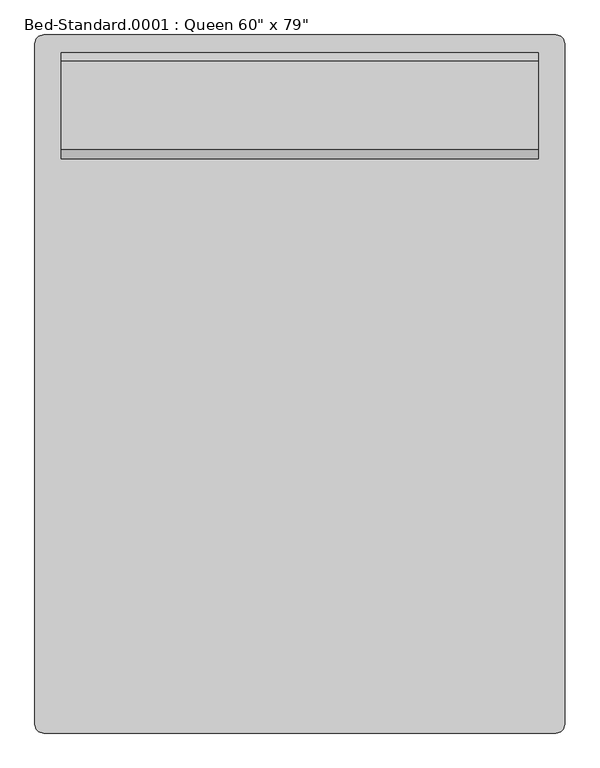
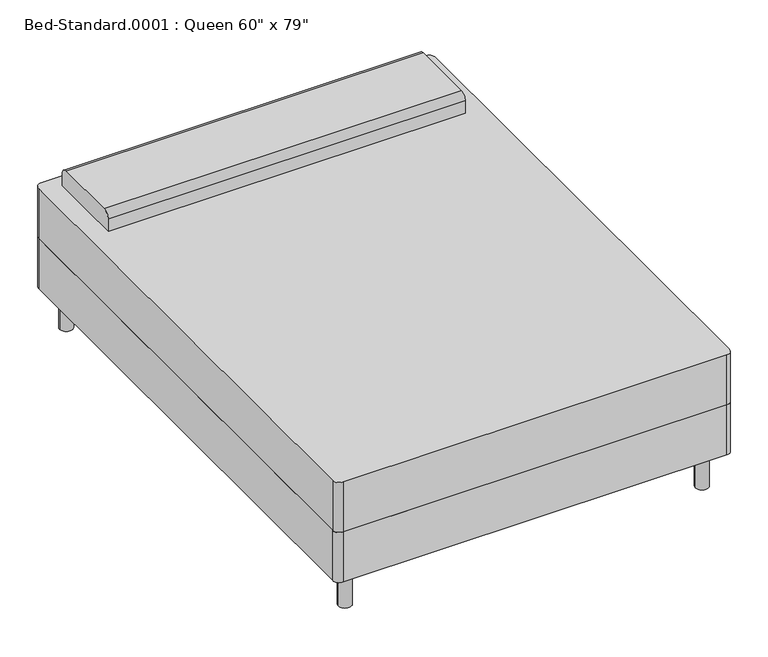
"""IFC4 building model written with IfcOpenShell, lengths in millimetres: furniture geometry."""

from ifc_helpers import new_model, si_unit, point, frame, frame_2d, origin, origin_with_axes, place, context, project, spatial, polyline, circle_curve, trimmed, segment, composite_curve, outline, extrude, source, transform, mapped, element, save


def furniture_e1791683(model_context):
    return source(origin(), model_context, "Body", "SweptSolid", [
        extrude(outline(composite_curve([segment(polyline([(-490.5114754, -1023.495082), (-490.5114754, 932.304918)]), True, "CONTINUOUS"), segment(trimmed(circle_curve(frame_2d((-465.1114754, 932.304918)), 25.4), [point((-490.5114754, 932.304918))], [point((-465.1114754, 957.704918))], False, "CARTESIAN"), True, "CONTINUOUS"), segment(polyline([(-465.1114754, 957.704918), (1008.0885246, 957.704918)]), True, "CONTINUOUS"), segment(trimmed(circle_curve(frame_2d((1008.0885246, 932.304918)), 25.4), [point((1008.0885246, 957.704918))], [point((1033.4885246, 932.304918))], False, "CARTESIAN"), True, "CONTINUOUS"), segment(polyline([(1033.4885246, 932.304918), (1033.4885246, -1023.495082)]), True, "CONTINUOUS"), segment(trimmed(circle_curve(frame_2d((1008.0885246, -1023.495082)), 25.4), [point((1033.4885246, -1023.495082))], [point((1008.0885246, -1048.895082))], False, "CARTESIAN"), True, "CONTINUOUS"), segment(polyline([(1008.0885246, -1048.895082), (-465.1114754, -1048.895082)]), True, "CONTINUOUS"), segment(trimmed(circle_curve(frame_2d((-465.1114754, -1023.495082)), 25.4), [point((-465.1114754, -1048.895082))], [point((-490.5114754, -1023.495082))], False, "CARTESIAN"), True, "CONTINUOUS")], self_intersect=False)), frame((0.0, 0.0, 152.4), z_axis=(0.0, 0.0, 1.0), x_axis=(1.0, 0.0, 0.0)), (0.0, 0.0, 1.0), 203.2),
        extrude(outline(composite_curve([segment(polyline([(602.104918, 558.8), (602.104918, 609.6)]), True, "CONTINUOUS"), segment(trimmed(circle_curve(frame_2d((627.504918, 609.6)), 25.4), [point((602.104918, 609.6))], [point((627.504918, 635.0))], False, "CARTESIAN"), True, "CONTINUOUS"), segment(polyline([(627.504918, 635.0), (881.504918, 635.0)]), True, "CONTINUOUS"), segment(trimmed(circle_curve(frame_2d((881.504918, 609.6)), 25.4), [point((881.504918, 635.0))], [point((906.904918, 609.6))], False, "CARTESIAN"), True, "CONTINUOUS"), segment(polyline([(906.904918, 609.6), (906.904918, 558.8), (602.104918, 558.8)]), True, "CONTINUOUS")], self_intersect=False)), frame((-414.3114754, 0.0, 0.0), z_axis=(1.0, 0.0, 0.0), x_axis=(0.0, 1.0, 0.0)), (0.0, 0.0, 1.0), 1371.6),
        extrude(outline(composite_curve([segment(trimmed(circle_curve(frame_2d((-414.3114754, 881.504918)), 25.4), [point((-439.7114754, 881.504918))], [point((-388.9114754, 881.504918))], False, "CARTESIAN"), True, "CONTINUOUS"), segment(trimmed(circle_curve(frame_2d((-414.3114754, 881.504918)), 25.4), [point((-388.9114754, 881.504918))], [point((-439.7114754, 881.504918))], False, "CARTESIAN"), True, "CONTINUOUS")], self_intersect=False)), origin_with_axes(), (0.0, 0.0, 1.0), 152.4),
        extrude(outline(composite_curve([segment(trimmed(circle_curve(frame_2d((957.2885246, 881.504918)), 25.4), [point((931.8885246, 881.504918))], [point((982.6885246, 881.504918))], False, "CARTESIAN"), True, "CONTINUOUS"), segment(trimmed(circle_curve(frame_2d((957.2885246, 881.504918)), 25.4), [point((982.6885246, 881.504918))], [point((931.8885246, 881.504918))], False, "CARTESIAN"), True, "CONTINUOUS")], self_intersect=False)), origin_with_axes(), (0.0, 0.0, 1.0), 152.4),
        extrude(outline(composite_curve([segment(trimmed(circle_curve(frame_2d((957.2885246, -972.695082)), 25.4), [point((931.8885246, -972.695082))], [point((982.6885246, -972.695082))], False, "CARTESIAN"), True, "CONTINUOUS"), segment(trimmed(circle_curve(frame_2d((957.2885246, -972.695082)), 25.4), [point((982.6885246, -972.695082))], [point((931.8885246, -972.695082))], False, "CARTESIAN"), True, "CONTINUOUS")], self_intersect=False)), origin_with_axes(), (0.0, 0.0, 1.0), 152.4),
        extrude(outline(composite_curve([segment(trimmed(circle_curve(frame_2d((-414.3114754, -972.695082)), 25.4), [point((-439.7114754, -972.695082))], [point((-388.9114754, -972.695082))], False, "CARTESIAN"), True, "CONTINUOUS"), segment(trimmed(circle_curve(frame_2d((-414.3114754, -972.695082)), 25.4), [point((-388.9114754, -972.695082))], [point((-439.7114754, -972.695082))], False, "CARTESIAN"), True, "CONTINUOUS")], self_intersect=False)), origin_with_axes(), (0.0, 0.0, 1.0), 152.4),
        extrude(outline(composite_curve([segment(polyline([(-465.1114754, 957.704918), (1008.0885246, 957.704918)]), True, "CONTINUOUS"), segment(trimmed(circle_curve(frame_2d((1008.0885246, 932.304918)), 25.4), [point((1008.0885246, 957.704918))], [point((1033.4885246, 932.304918))], False, "CARTESIAN"), True, "CONTINUOUS"), segment(polyline([(1033.4885246, 932.304918), (1033.4885246, -1023.495082)]), True, "CONTINUOUS"), segment(trimmed(circle_curve(frame_2d((1008.0885246, -1023.495082)), 25.4), [point((1033.4885246, -1023.495082))], [point((1008.0885246, -1048.895082))], False, "CARTESIAN"), True, "CONTINUOUS"), segment(polyline([(1008.0885246, -1048.895082), (-465.1114754, -1048.895082)]), True, "CONTINUOUS"), segment(trimmed(circle_curve(frame_2d((-465.1114754, -1023.495082)), 25.4), [point((-465.1114754, -1048.895082))], [point((-490.5114754, -1023.495082))], False, "CARTESIAN"), True, "CONTINUOUS"), segment(polyline([(-490.5114754, -1023.495082), (-490.5114754, 932.304918)]), True, "CONTINUOUS"), segment(trimmed(circle_curve(frame_2d((-465.1114754, 932.304918)), 25.4), [point((-490.5114754, 932.304918))], [point((-465.1114754, 957.704918))], False, "CARTESIAN"), True, "CONTINUOUS")], self_intersect=False)), frame((0.0, 0.0, 355.6), z_axis=(0.0, 0.0, 1.0), x_axis=(1.0, 0.0, 0.0)), (0.0, 0.0, 1.0), 203.2),
    ])


if __name__ == "__main__":
    model = new_model("IFC4")
    model_context = context("Model", 3, world=origin())
    ifc_project = project(units=[si_unit("LENGTHUNIT", "METRE", prefix="MILLI")], contexts=[model_context])
    site = spatial("IfcSite", under=ifc_project)
    building = spatial("IfcBuilding", under=site)
    placement = place(None, origin())
    furniture_shape = furniture_e1791683(model_context)
    element("IfcFurniture", 1, ObjectType="Bed-Standard.0001 : Queen 60\" x 79\"", at=placement, inside=building, context=model_context, shape_type="MappedRepresentation", body=[
        mapped(furniture_shape, transform((0.0, 0.0, 0.0), x_axis=(1.0, 0.0, 0.0), y_axis=(0.0, 1.0, 0.0), z_axis=(0.0, 0.0, 1.0))),
    ])
    save(model, "model.ifc")

# Revit data of these elements
# Type "Bed-Standard.0001 : Queen 60\" x 79\""
#   Assembly Code = "E2020200"
#   Length = 6' - 7"
#   Width = 5' - 0"
#   Leg Material = Steel, Chrome Plated
#   Mattress Material = Linen, White
#   Default Elevation = 0
# Element 1 (IfcFurniture, "Bed-Standard.0001 : Queen 60\" x 79\"")
#   Materials on its faces: "Linen, White", "Steel, Chrome Plated"
# Materials
#   "Steel, Chrome Plated": class "Metal", colour RGB 17 17 17, transparency 0, Description = "Chromiuim plated steel", Cost = 0
#   "Linen, White": class "Textile", colour RGB 247 247 239, transparency 0, Description = "Linen, white", Cost = 0
